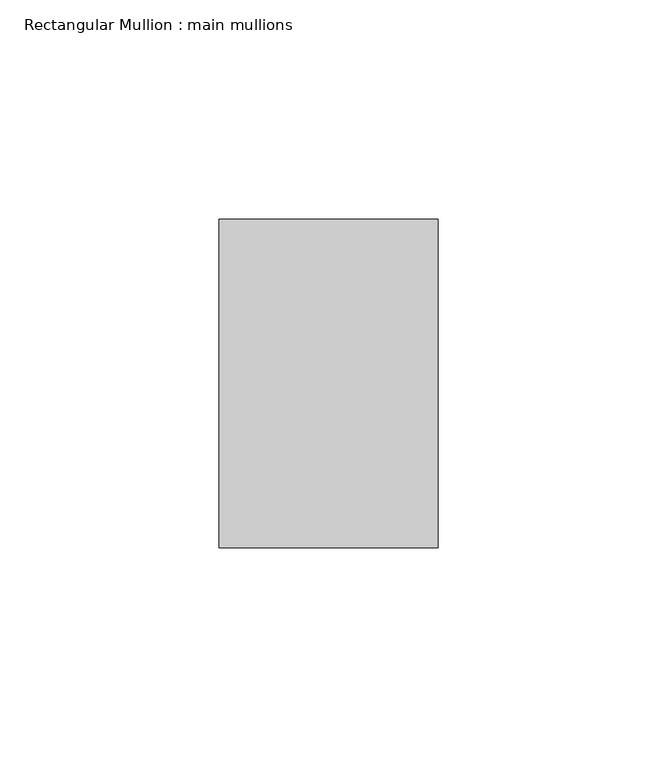
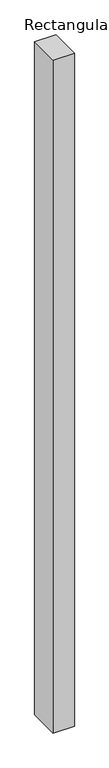
"""IFC4 building model written with IfcOpenShell, lengths in millimetres: member geometry, Rectangular Mullion : main mullions."""

from ifc_helpers import new_model, si_unit, frame, origin, place, context, project, spatial, polyline, outline, extrude, source, transform, mapped, element, save


def rectangular_mullion_main_mullions_5bed117f(model_context):
    return source(origin(), model_context, "Body", "SweptSolid", [
        extrude(outline(polyline([(0.0, 37.5), (0.0, -37.5), (-50.0, -37.5), (-50.0, 37.5), (0.0, 37.5)])), frame((0.0, 0.0, -1675.0), z_axis=(0.0, 0.0, 1.0), x_axis=(1.0, 0.0, 0.0)), (0.0, 0.0, 1.0), 1675.0),
    ])


if __name__ == "__main__":
    model = new_model("IFC4")
    model_context = context("Model", 3, world=origin())
    ifc_project = project(units=[si_unit("LENGTHUNIT", "METRE", prefix="MILLI")], contexts=[model_context])
    site = spatial("IfcSite", under=ifc_project)
    building = spatial("IfcBuilding", under=site)
    placement = place(None, origin())
    rectangular_mullion_main_mullions_shape = rectangular_mullion_main_mullions_5bed117f(model_context)
    element("IfcMember", 1, ObjectType="Rectangular Mullion : main mullions", at=placement, inside=building, context=model_context, shape_type="MappedRepresentation", body=[
        mapped(rectangular_mullion_main_mullions_shape, transform((0.0, 0.0, 0.0), x_axis=(1.0, 0.0, 0.0), y_axis=(0.0, 1.0, 0.0), z_axis=(0.0, 0.0, 1.0))),
    ])
    save(model, "model.ifc")

# Revit data of these elements
# Type "Rectangular Mullion : main mullions"
#   built-in parameter 1007304 = 0.246063 (stored number, unit not read)
#   built-in parameter 1007301 = 0.082021 (stored number, unit not read)
#   built-in parameter 1007300 = 0.082021 (stored number, unit not read)
# Element 1 (IfcMember, "Rectangular Mullion : main mullions")
#   Materials on its faces: "Aluminum"
# Materials
#   "Aluminum": class "Metal", colour RGB 136 136 136, transparency 0, Description = "Aluminum 6061", Cost = 0
